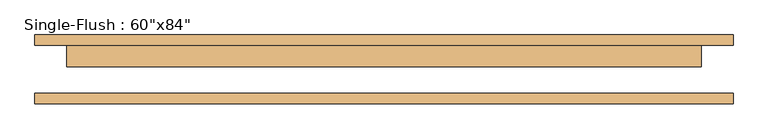
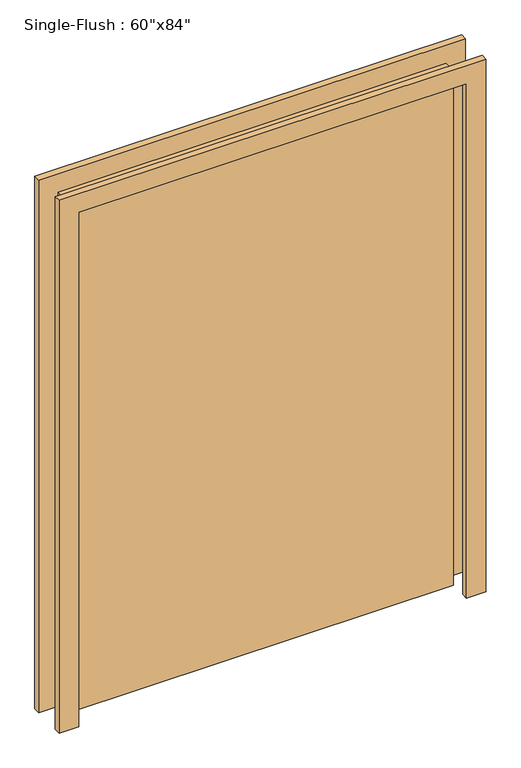
"""IFC4 building model written with IfcOpenShell, lengths in millimetres: door geometry."""

from ifc_helpers import new_model, si_unit, frame, origin, origin_with_axes, place, context, project, spatial, polyline, outline, extrude, source, transform, mapped, element, save


def door_ea54c7da(model_context):
    return source(origin(), model_context, "Body", "SweptSolid", [
        extrude(outline(polyline([(2209.8, -838.2), (0.0, -838.2), (0.0, -762.0), (2133.6, -762.0), (2133.6, 762.0), (0.0, 762.0), (0.0, 838.2), (2209.8, 838.2), (2209.8, -838.2)])), frame((0.0, 57.15, 0.0), z_axis=(0.0, 1.0, 0.0), x_axis=(0.0, 0.0, 1.0)), (0.0, 0.0, 1.0), 25.4),
        extrude(outline(polyline([(2209.8, 838.2), (2209.8, -838.2), (0.0, -838.2), (0.0, -762.0), (2133.6, -762.0), (2133.6, 762.0), (0.0, 762.0), (0.0, 838.2), (2209.8, 838.2)])), frame((0.0, -82.55, 0.0), z_axis=(0.0, 1.0, 0.0), x_axis=(0.0, 0.0, 1.0)), (0.0, 0.0, 1.0), 25.4),
        extrude(outline(polyline([(762.0, 6.35), (-762.0, 6.35), (-762.0, 57.15), (762.0, 57.15), (762.0, 6.35)])), origin_with_axes(), (0.0, 0.0, 1.0), 2133.6),
    ])


if __name__ == "__main__":
    model = new_model("IFC4")
    model_context = context("Model", 3, world=origin())
    ifc_project = project(units=[si_unit("LENGTHUNIT", "METRE", prefix="MILLI")], contexts=[model_context])
    site = spatial("IfcSite", under=ifc_project)
    building = spatial("IfcBuilding", under=site)
    placement = place(None, origin())
    door_shape = door_ea54c7da(model_context)
    element("IfcDoor", 1, ObjectType="Single-Flush : 60\"x84\"", at=placement, inside=building, context=model_context, shape_type="MappedRepresentation", body=[
        mapped(door_shape, transform((0.0, 0.0, 0.0), x_axis=(1.0, 0.0, 0.0), y_axis=(0.0, 1.0, 0.0), z_axis=(0.0, 0.0, 1.0))),
    ])
    save(model, "model.ifc")

# Revit data of these elements
# Type "Single-Flush : 60\"x84\""
#   Type Mark = "8"
#   Construction Type Id = "MDOOR"
#   Assembly Code = "C1020"
#   Analytic Construction = "Metal"
#   Thickness = 0' - 2"
#   Heat Transfer Coefficient (U) = 0.651978 BTU/(h·ft²·°F)
#   Height = 7' - 0"
#   Trim Projection Ext = 0' - 1"
#   Trim Projection Int = 0' - 1"
#   Trim Width = 0' - 3"
#   Width = 5' - 0"
#   Define Thermal Properties by = 1
#   Door Material = Door - Panel
#   Frame Material = Door - Frame
#   Visual Light Transmittance = 0
#   Solar Heat Gain Coefficient = 0
#   Function = (empty or 0)
#   Wall Closure = (empty or 0)
# Element 1 (IfcDoor, "Single-Flush : 60\"x84\"")
#   Materials on its faces: "Door - Frame", "Door - Panel"
# Materials
#   "Door - Panel": class "Wood", colour RGB 210 159 95, transparency 0, Cost = 0
#   "Door - Frame": colour RGB 118 70 51, transparency 0, Cost = 0
